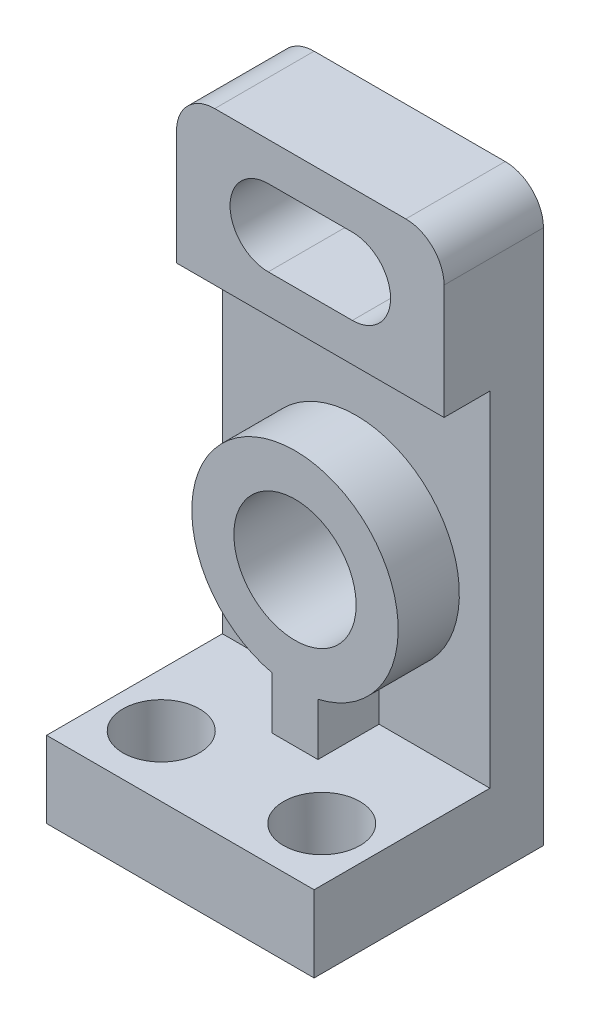
ISO-10303-21;
HEADER;
FILE_DESCRIPTION(('STEP AP214'),'2;1');
FILE_NAME('part.step','',(''),(''),'','','');
FILE_SCHEMA(('AUTOMOTIVE_DESIGN { 1 0 10303 214 1 1 1 1 }'));
ENDSEC;
DATA;
#1=APPLICATION_CONTEXT('core data for automotive mechanical design processes');
#2=APPLICATION_PROTOCOL_DEFINITION('international standard','automotive_design',2000,#1);
#3=PRODUCT_CONTEXT('',#1,'mechanical');
#4=PRODUCT('Part','Part','',(#3));
#5=PRODUCT_RELATED_PRODUCT_CATEGORY('part','',(#4));
#6=PRODUCT_DEFINITION_FORMATION('','',#4);
#7=PRODUCT_DEFINITION_CONTEXT('part definition',#1,'design');
#8=PRODUCT_DEFINITION('design','',#6,#7);
#9=PRODUCT_DEFINITION_SHAPE('','',#8);
#10=(LENGTH_UNIT() NAMED_UNIT(*) SI_UNIT(.MILLI.,.METRE.));
#11=(NAMED_UNIT(*) PLANE_ANGLE_UNIT() SI_UNIT($,.RADIAN.));
#12=(NAMED_UNIT(*) SI_UNIT($,.STERADIAN.) SOLID_ANGLE_UNIT());
#13=UNCERTAINTY_MEASURE_WITH_UNIT(LENGTH_MEASURE(1.E-05),#10,'distance_accuracy_value','');
#14=(GEOMETRIC_REPRESENTATION_CONTEXT(3) GLOBAL_UNCERTAINTY_ASSIGNED_CONTEXT((#13)) GLOBAL_UNIT_ASSIGNED_CONTEXT((#10,
#11,#12)) REPRESENTATION_CONTEXT('',''));
#15=CARTESIAN_POINT('',(0.,0.,0.));
#16=DIRECTION('',(0.,0.,1.));
#17=DIRECTION('',(1.,0.,0.));
#18=AXIS2_PLACEMENT_3D('',#15,#16,#17);
#19=CARTESIAN_POINT('',(17.5,10.,6.99999999999999));
#20=DIRECTION('',(0.,0.,-1.));
#21=DIRECTION('',(-1.,0.,0.));
#22=AXIS2_PLACEMENT_3D('',#19,#20,#21);
#23=PLANE('',#22);
#24=DIRECTION('',(0.,-1.,0.));
#25=VECTOR('',#24,1.);
#26=CARTESIAN_POINT('',(-3.,16.8375534189118,6.99999999999999));
#27=LINE('',#26,#25);
#28=CARTESIAN_POINT('',(-3.,16.8375534189118,6.99999999999999));
#29=VERTEX_POINT('',#28);
#30=CARTESIAN_POINT('',(-3.,10.,6.99999999999999));
#31=VERTEX_POINT('',#30);
#32=EDGE_CURVE('E211',#29,#31,#27,.T.);
#33=ORIENTED_EDGE('',*,*,#32,.F.);
#34=CARTESIAN_POINT('',(0.,30.,6.99999999999999));
#35=DIRECTION('',(0.,0.,1.));
#36=DIRECTION('',(1.,0.,0.));
#37=AXIS2_PLACEMENT_3D('',#34,#35,#36);
#38=CIRCLE('',#37,13.5);
#39=CARTESIAN_POINT('',(3.,16.8375534189118,6.99999999999999));
#40=VERTEX_POINT('',#39);
#41=EDGE_CURVE('E167',#40,#29,#38,.T.);
#42=ORIENTED_EDGE('',*,*,#41,.F.);
#43=DIRECTION('',(0.,1.,0.));
#44=VECTOR('',#43,1.);
#45=CARTESIAN_POINT('',(3.,16.8375534189118,6.99999999999999));
#46=LINE('',#45,#44);
#47=CARTESIAN_POINT('',(3.,10.,6.99999999999999));
#48=VERTEX_POINT('',#47);
#49=EDGE_CURVE('E203',#48,#40,#46,.T.);
#50=ORIENTED_EDGE('',*,*,#49,.F.);
#51=DIRECTION('',(-1.,0.,0.));
#52=VECTOR('',#51,1.);
#53=CARTESIAN_POINT('',(17.5,10.,6.99999999999999));
#54=LINE('',#53,#52);
#55=CARTESIAN_POINT('',(17.5,10.,6.99999999999999));
#56=VERTEX_POINT('',#55);
#57=EDGE_CURVE('E262',#56,#48,#54,.T.);
#58=ORIENTED_EDGE('',*,*,#57,.F.);
#59=DIRECTION('',(0.,-1.,0.));
#60=VECTOR('',#59,1.);
#61=CARTESIAN_POINT('',(17.5,10.,6.99999999999999));
#62=LINE('',#61,#60);
#63=CARTESIAN_POINT('',(17.5,55.,6.99999999999999));
#64=VERTEX_POINT('',#63);
#65=EDGE_CURVE('E235',#64,#56,#62,.T.);
#66=ORIENTED_EDGE('',*,*,#65,.F.);
#67=DIRECTION('',(-1.,0.,0.));
#68=VECTOR('',#67,1.);
#69=CARTESIAN_POINT('',(17.5,55.,6.99999999999999));
#70=LINE('',#69,#68);
#71=CARTESIAN_POINT('',(-17.5,55.,6.99999999999999));
#72=VERTEX_POINT('',#71);
#73=EDGE_CURVE('E270',#64,#72,#70,.T.);
#74=ORIENTED_EDGE('',*,*,#73,.T.);
#75=DIRECTION('',(0.,-1.,0.));
#76=VECTOR('',#75,1.);
#77=CARTESIAN_POINT('',(-17.5,10.,6.99999999999999));
#78=LINE('',#77,#76);
#79=CARTESIAN_POINT('',(-17.5,10.,6.99999999999999));
#80=VERTEX_POINT('',#79);
#81=EDGE_CURVE('E250',#72,#80,#78,.T.);
#82=ORIENTED_EDGE('',*,*,#81,.T.);
#83=EDGE_CURVE('E263',#31,#80,#54,.T.);
#84=ORIENTED_EDGE('',*,*,#83,.F.);
#85=EDGE_LOOP('',(#33,#42,#50,#58,#66,#74,#82,#84));
#86=FACE_BOUND('',#85,.T.);
#87=ADVANCED_FACE('F39',(#86),#23,.F.);
#88=CARTESIAN_POINT('',(17.5,10.,30.));
#89=DIRECTION('',(0.,-1.,0.));
#90=DIRECTION('',(0.,0.,-1.));
#91=AXIS2_PLACEMENT_3D('',#88,#89,#90);
#92=PLANE('',#91);
#93=CARTESIAN_POINT('',(-10.5,10.,22.));
#94=DIRECTION('',(0.,1.,0.));
#95=DIRECTION('',(0.,0.,1.));
#96=AXIS2_PLACEMENT_3D('',#93,#94,#95);
#97=CIRCLE('',#96,5.);
#98=CARTESIAN_POINT('',(-10.5,10.,27.));
#99=VERTEX_POINT('',#98);
#100=EDGE_CURVE('E314',#99,#99,#97,.T.);
#101=ORIENTED_EDGE('',*,*,#100,.F.);
#102=EDGE_LOOP('',(#101));
#103=FACE_BOUND('',#102,.T.);
#104=CARTESIAN_POINT('',(10.5,10.,22.));
#105=DIRECTION('',(0.,1.,0.));
#106=DIRECTION('',(0.,0.,-1.));
#107=AXIS2_PLACEMENT_3D('',#104,#105,#106);
#108=CIRCLE('',#107,5.);
#109=CARTESIAN_POINT('',(10.5,10.,17.));
#110=VERTEX_POINT('',#109);
#111=EDGE_CURVE('E312',#110,#110,#108,.T.);
#112=ORIENTED_EDGE('',*,*,#111,.F.);
#113=EDGE_LOOP('',(#112));
#114=FACE_BOUND('',#113,.T.);
#115=DIRECTION('',(0.,0.,-1.));
#116=VECTOR('',#115,1.);
#117=CARTESIAN_POINT('',(-3.,10.,15.));
#118=LINE('',#117,#116);
#119=CARTESIAN_POINT('',(-3.,10.,15.));
#120=VERTEX_POINT('',#119);
#121=EDGE_CURVE('E217',#120,#31,#118,.T.);
#122=ORIENTED_EDGE('',*,*,#121,.T.);
#123=ORIENTED_EDGE('',*,*,#83,.T.);
#124=DIRECTION('',(0.,0.,1.));
#125=VECTOR('',#124,1.);
#126=CARTESIAN_POINT('',(-17.5,10.,30.));
#127=LINE('',#126,#125);
#128=CARTESIAN_POINT('',(-17.5,10.,30.));
#129=VERTEX_POINT('',#128);
#130=EDGE_CURVE('E246',#80,#129,#127,.T.);
#131=ORIENTED_EDGE('',*,*,#130,.T.);
#132=DIRECTION('',(-1.,0.,0.));
#133=VECTOR('',#132,1.);
#134=CARTESIAN_POINT('',(17.5,10.,30.));
#135=LINE('',#134,#133);
#136=CARTESIAN_POINT('',(17.5,10.,30.));
#137=VERTEX_POINT('',#136);
#138=EDGE_CURVE('E257',#137,#129,#135,.T.);
#139=ORIENTED_EDGE('',*,*,#138,.F.);
#140=DIRECTION('',(0.,0.,1.));
#141=VECTOR('',#140,1.);
#142=CARTESIAN_POINT('',(17.5,10.,30.));
#143=LINE('',#142,#141);
#144=EDGE_CURVE('E234',#56,#137,#143,.T.);
#145=ORIENTED_EDGE('',*,*,#144,.F.);
#146=ORIENTED_EDGE('',*,*,#57,.T.);
#147=DIRECTION('',(0.,0.,-1.));
#148=VECTOR('',#147,1.);
#149=CARTESIAN_POINT('',(3.,10.,15.));
#150=LINE('',#149,#148);
#151=CARTESIAN_POINT('',(3.,10.,15.));
#152=VERTEX_POINT('',#151);
#153=EDGE_CURVE('E216',#152,#48,#150,.T.);
#154=ORIENTED_EDGE('',*,*,#153,.F.);
#155=DIRECTION('',(1.,0.,0.));
#156=VECTOR('',#155,1.);
#157=CARTESIAN_POINT('',(-3.,10.,15.));
#158=LINE('',#157,#156);
#159=EDGE_CURVE('E204',#120,#152,#158,.T.);
#160=ORIENTED_EDGE('',*,*,#159,.F.);
#161=EDGE_LOOP('',(#122,#123,#131,#139,#145,#146,#154,#160));
#162=FACE_BOUND('',#161,.T.);
#163=ADVANCED_FACE('F324',(#103,#114,#162),#92,.F.);
#164=CARTESIAN_POINT('',(17.5,75.,0.));
#165=DIRECTION('',(0.,0.,1.));
#166=DIRECTION('',(0.,-1.,0.));
#167=AXIS2_PLACEMENT_3D('',#164,#165,#166);
#168=PLANE('',#167);
#169=DIRECTION('',(1.,0.,0.));
#170=VECTOR('',#169,1.);
#171=CARTESIAN_POINT('',(-5.5,70.,0.));
#172=LINE('',#171,#170);
#173=CARTESIAN_POINT('',(-5.5,70.,0.));
#174=VERTEX_POINT('',#173);
#175=CARTESIAN_POINT('',(5.5,70.,0.));
#176=VERTEX_POINT('',#175);
#177=EDGE_CURVE('E179',#174,#176,#172,.T.);
#178=ORIENTED_EDGE('',*,*,#177,.F.);
#179=CARTESIAN_POINT('',(-5.5,65.,0.));
#180=DIRECTION('',(0.,0.,1.));
#181=DIRECTION('',(0.,-1.,0.));
#182=AXIS2_PLACEMENT_3D('',#179,#180,#181);
#183=CIRCLE('',#182,5.);
#184=CARTESIAN_POINT('',(-5.5,60.,0.));
#185=VERTEX_POINT('',#184);
#186=EDGE_CURVE('E170',#185,#174,#183,.F.);
#187=ORIENTED_EDGE('',*,*,#186,.F.);
#188=DIRECTION('',(-1.,0.,0.));
#189=VECTOR('',#188,1.);
#190=CARTESIAN_POINT('',(-5.5,60.,0.));
#191=LINE('',#190,#189);
#192=CARTESIAN_POINT('',(5.5,60.,0.));
#193=VERTEX_POINT('',#192);
#194=EDGE_CURVE('E161',#193,#185,#191,.T.);
#195=ORIENTED_EDGE('',*,*,#194,.F.);
#196=CARTESIAN_POINT('',(5.5,65.,0.));
#197=DIRECTION('',(0.,0.,1.));
#198=DIRECTION('',(0.,-1.,0.));
#199=AXIS2_PLACEMENT_3D('',#196,#197,#198);
#200=CIRCLE('',#199,5.);
#201=EDGE_CURVE('E182',#176,#193,#200,.F.);
#202=ORIENTED_EDGE('',*,*,#201,.F.);
#203=EDGE_LOOP('',(#178,#187,#195,#202));
#204=FACE_BOUND('',#203,.T.);
#205=CARTESIAN_POINT('',(0.,30.,0.));
#206=DIRECTION('',(0.,0.,1.));
#207=DIRECTION('',(0.,-1.,0.));
#208=AXIS2_PLACEMENT_3D('',#205,#206,#207);
#209=CIRCLE('',#208,8.);
#210=CARTESIAN_POINT('',(0.,22.,0.));
#211=VERTEX_POINT('',#210);
#212=EDGE_CURVE('E173',#211,#211,#209,.F.);
#213=ORIENTED_EDGE('',*,*,#212,.F.);
#214=EDGE_LOOP('',(#213));
#215=FACE_BOUND('',#214,.T.);
#216=DIRECTION('',(-1.,0.,0.));
#217=VECTOR('',#216,1.);
#218=CARTESIAN_POINT('',(17.5,75.,0.));
#219=LINE('',#218,#217);
#220=CARTESIAN_POINT('',(12.5,75.,0.));
#221=VERTEX_POINT('',#220);
#222=CARTESIAN_POINT('',(-12.5,75.,0.));
#223=VERTEX_POINT('',#222);
#224=EDGE_CURVE('E277',#221,#223,#219,.T.);
#225=ORIENTED_EDGE('',*,*,#224,.F.);
#226=CARTESIAN_POINT('',(12.5,70.,0.));
#227=DIRECTION('',(0.,0.,1.));
#228=DIRECTION('',(0.,-1.,0.));
#229=AXIS2_PLACEMENT_3D('',#226,#227,#228);
#230=CIRCLE('',#229,5.);
#231=CARTESIAN_POINT('',(17.5,70.,0.));
#232=VERTEX_POINT('',#231);
#233=EDGE_CURVE('E291',#221,#232,#230,.F.);
#234=ORIENTED_EDGE('',*,*,#233,.T.);
#235=DIRECTION('',(0.,1.,0.));
#236=VECTOR('',#235,1.);
#237=CARTESIAN_POINT('',(17.5,75.,0.));
#238=LINE('',#237,#236);
#239=CARTESIAN_POINT('',(17.5,0.,0.));
#240=VERTEX_POINT('',#239);
#241=EDGE_CURVE('E221',#240,#232,#238,.T.);
#242=ORIENTED_EDGE('',*,*,#241,.F.);
#243=DIRECTION('',(-1.,0.,0.));
#244=VECTOR('',#243,1.);
#245=CARTESIAN_POINT('',(17.5,0.,0.));
#246=LINE('',#245,#244);
#247=CARTESIAN_POINT('',(-17.5,0.,0.));
#248=VERTEX_POINT('',#247);
#249=EDGE_CURVE('E238',#240,#248,#246,.T.);
#250=ORIENTED_EDGE('',*,*,#249,.T.);
#251=DIRECTION('',(0.,1.,0.));
#252=VECTOR('',#251,1.);
#253=CARTESIAN_POINT('',(-17.5,75.,0.));
#254=LINE('',#253,#252);
#255=CARTESIAN_POINT('',(-17.5,70.,0.));
#256=VERTEX_POINT('',#255);
#257=EDGE_CURVE('E224',#248,#256,#254,.T.);
#258=ORIENTED_EDGE('',*,*,#257,.T.);
#259=CARTESIAN_POINT('',(-12.5,70.,0.));
#260=DIRECTION('',(0.,0.,1.));
#261=DIRECTION('',(0.,-1.,0.));
#262=AXIS2_PLACEMENT_3D('',#259,#260,#261);
#263=CIRCLE('',#262,5.);
#264=EDGE_CURVE('E292',#256,#223,#263,.F.);
#265=ORIENTED_EDGE('',*,*,#264,.T.);
#266=EDGE_LOOP('',(#225,#234,#242,#250,#258,#265));
#267=FACE_BOUND('',#266,.T.);
#268=ADVANCED_FACE('F180',(#204,#215,#267),#168,.F.);
#269=CARTESIAN_POINT('',(17.5,75.,13.));
#270=DIRECTION('',(0.,-1.,0.));
#271=DIRECTION('',(0.,0.,-1.));
#272=AXIS2_PLACEMENT_3D('',#269,#270,#271);
#273=PLANE('',#272);
#274=DIRECTION('',(-1.,0.,0.));
#275=VECTOR('',#274,1.);
#276=CARTESIAN_POINT('',(17.5,75.,13.));
#277=LINE('',#276,#275);
#278=CARTESIAN_POINT('',(12.5,75.,13.));
#279=VERTEX_POINT('',#278);
#280=CARTESIAN_POINT('',(-12.5,75.,13.));
#281=VERTEX_POINT('',#280);
#282=EDGE_CURVE('E272',#279,#281,#277,.T.);
#283=ORIENTED_EDGE('',*,*,#282,.F.);
#284=DIRECTION('',(0.,0.,1.));
#285=VECTOR('',#284,1.);
#286=CARTESIAN_POINT('',(12.5,75.,13.));
#287=LINE('',#286,#285);
#288=EDGE_CURVE('E289',#279,#221,#287,.F.);
#289=ORIENTED_EDGE('',*,*,#288,.T.);
#290=ORIENTED_EDGE('',*,*,#224,.T.);
#291=DIRECTION('',(0.,0.,1.));
#292=VECTOR('',#291,1.);
#293=CARTESIAN_POINT('',(-12.5,75.,13.));
#294=LINE('',#293,#292);
#295=EDGE_CURVE('E287',#223,#281,#294,.T.);
#296=ORIENTED_EDGE('',*,*,#295,.T.);
#297=EDGE_LOOP('',(#283,#289,#290,#296));
#298=FACE_BOUND('',#297,.T.);
#299=ADVANCED_FACE('F392',(#298),#273,.F.);
#300=CARTESIAN_POINT('',(17.5,55.,13.));
#301=DIRECTION('',(0.,0.,-1.));
#302=DIRECTION('',(-1.,0.,0.));
#303=AXIS2_PLACEMENT_3D('',#300,#301,#302);
#304=PLANE('',#303);
#305=DIRECTION('',(-1.,0.,0.));
#306=VECTOR('',#305,1.);
#307=CARTESIAN_POINT('',(17.5,60.,13.));
#308=LINE('',#307,#306);
#309=CARTESIAN_POINT('',(5.5,60.,13.));
#310=VERTEX_POINT('',#309);
#311=CARTESIAN_POINT('',(-5.5,60.,13.));
#312=VERTEX_POINT('',#311);
#313=EDGE_CURVE('E297',#310,#312,#308,.T.);
#314=ORIENTED_EDGE('',*,*,#313,.T.);
#315=CARTESIAN_POINT('',(-5.5,65.,13.));
#316=DIRECTION('',(0.,0.,-1.));
#317=DIRECTION('',(-1.,0.,0.));
#318=AXIS2_PLACEMENT_3D('',#315,#316,#317);
#319=CIRCLE('',#318,5.);
#320=CARTESIAN_POINT('',(-5.5,70.,13.));
#321=VERTEX_POINT('',#320);
#322=EDGE_CURVE('E11',#312,#321,#319,.T.);
#323=ORIENTED_EDGE('',*,*,#322,.T.);
#324=DIRECTION('',(1.,0.,0.));
#325=VECTOR('',#324,1.);
#326=CARTESIAN_POINT('',(17.5,70.,13.));
#327=LINE('',#326,#325);
#328=CARTESIAN_POINT('',(5.5,70.,13.));
#329=VERTEX_POINT('',#328);
#330=EDGE_CURVE('E50',#321,#329,#327,.T.);
#331=ORIENTED_EDGE('',*,*,#330,.T.);
#332=CARTESIAN_POINT('',(5.5,65.,13.));
#333=DIRECTION('',(0.,0.,-1.));
#334=DIRECTION('',(-1.,0.,0.));
#335=AXIS2_PLACEMENT_3D('',#332,#333,#334);
#336=CIRCLE('',#335,5.);
#337=EDGE_CURVE('E298',#329,#310,#336,.T.);
#338=ORIENTED_EDGE('',*,*,#337,.T.);
#339=EDGE_LOOP('',(#314,#323,#331,#338));
#340=FACE_BOUND('',#339,.T.);
#341=DIRECTION('',(0.,-1.,0.));
#342=VECTOR('',#341,1.);
#343=CARTESIAN_POINT('',(17.5,55.,13.));
#344=LINE('',#343,#342);
#345=CARTESIAN_POINT('',(17.5,70.,13.));
#346=VERTEX_POINT('',#345);
#347=CARTESIAN_POINT('',(17.5,55.,13.));
#348=VERTEX_POINT('',#347);
#349=EDGE_CURVE('E227',#346,#348,#344,.T.);
#350=ORIENTED_EDGE('',*,*,#349,.F.);
#351=CARTESIAN_POINT('',(12.5,70.,13.));
#352=DIRECTION('',(0.,0.,-1.));
#353=DIRECTION('',(-1.,0.,0.));
#354=AXIS2_PLACEMENT_3D('',#351,#352,#353);
#355=CIRCLE('',#354,5.);
#356=EDGE_CURVE('E283',#346,#279,#355,.F.);
#357=ORIENTED_EDGE('',*,*,#356,.T.);
#358=ORIENTED_EDGE('',*,*,#282,.T.);
#359=CARTESIAN_POINT('',(-12.5,70.,13.));
#360=DIRECTION('',(0.,0.,-1.));
#361=DIRECTION('',(-1.,0.,0.));
#362=AXIS2_PLACEMENT_3D('',#359,#360,#361);
#363=CIRCLE('',#362,5.);
#364=CARTESIAN_POINT('',(-17.5,70.,13.));
#365=VERTEX_POINT('',#364);
#366=EDGE_CURVE('E282',#281,#365,#363,.F.);
#367=ORIENTED_EDGE('',*,*,#366,.T.);
#368=DIRECTION('',(0.,-1.,0.));
#369=VECTOR('',#368,1.);
#370=CARTESIAN_POINT('',(-17.5,55.,13.));
#371=LINE('',#370,#369);
#372=CARTESIAN_POINT('',(-17.5,55.,13.));
#373=VERTEX_POINT('',#372);
#374=EDGE_CURVE('E244',#365,#373,#371,.T.);
#375=ORIENTED_EDGE('',*,*,#374,.T.);
#376=DIRECTION('',(-1.,0.,0.));
#377=VECTOR('',#376,1.);
#378=CARTESIAN_POINT('',(17.5,55.,13.));
#379=LINE('',#378,#377);
#380=EDGE_CURVE('E269',#348,#373,#379,.T.);
#381=ORIENTED_EDGE('',*,*,#380,.F.);
#382=EDGE_LOOP('',(#350,#357,#358,#367,#375,#381));
#383=FACE_BOUND('',#382,.T.);
#384=ADVANCED_FACE('F303',(#340,#383),#304,.F.);
#385=CARTESIAN_POINT('',(17.5,55.,6.99999999999999));
#386=DIRECTION('',(0.,1.,0.));
#387=DIRECTION('',(0.,0.,1.));
#388=AXIS2_PLACEMENT_3D('',#385,#386,#387);
#389=PLANE('',#388);
#390=DIRECTION('',(0.,0.,-1.));
#391=VECTOR('',#390,1.);
#392=CARTESIAN_POINT('',(-17.5,55.,6.99999999999999));
#393=LINE('',#392,#391);
#394=EDGE_CURVE('E245',#373,#72,#393,.T.);
#395=ORIENTED_EDGE('',*,*,#394,.T.);
#396=ORIENTED_EDGE('',*,*,#73,.F.);
#397=DIRECTION('',(0.,0.,-1.));
#398=VECTOR('',#397,1.);
#399=CARTESIAN_POINT('',(17.5,55.,6.99999999999999));
#400=LINE('',#399,#398);
#401=EDGE_CURVE('E230',#348,#64,#400,.T.);
#402=ORIENTED_EDGE('',*,*,#401,.F.);
#403=ORIENTED_EDGE('',*,*,#380,.T.);
#404=EDGE_LOOP('',(#395,#396,#402,#403));
#405=FACE_BOUND('',#404,.T.);
#406=ADVANCED_FACE('F387',(#405),#389,.F.);
#407=CARTESIAN_POINT('',(17.5,0.,30.));
#408=DIRECTION('',(0.,0.,-1.));
#409=DIRECTION('',(-1.,0.,0.));
#410=AXIS2_PLACEMENT_3D('',#407,#408,#409);
#411=PLANE('',#410);
#412=DIRECTION('',(0.,-1.,0.));
#413=VECTOR('',#412,1.);
#414=CARTESIAN_POINT('',(-17.5,0.,30.));
#415=LINE('',#414,#413);
#416=CARTESIAN_POINT('',(-17.5,0.,30.));
#417=VERTEX_POINT('',#416);
#418=EDGE_CURVE('E252',#129,#417,#415,.T.);
#419=ORIENTED_EDGE('',*,*,#418,.T.);
#420=DIRECTION('',(-1.,0.,0.));
#421=VECTOR('',#420,1.);
#422=CARTESIAN_POINT('',(17.5,0.,30.));
#423=LINE('',#422,#421);
#424=CARTESIAN_POINT('',(17.5,0.,30.));
#425=VERTEX_POINT('',#424);
#426=EDGE_CURVE('E260',#425,#417,#423,.T.);
#427=ORIENTED_EDGE('',*,*,#426,.F.);
#428=DIRECTION('',(0.,-1.,0.));
#429=VECTOR('',#428,1.);
#430=CARTESIAN_POINT('',(17.5,0.,30.));
#431=LINE('',#430,#429);
#432=EDGE_CURVE('E237',#137,#425,#431,.T.);
#433=ORIENTED_EDGE('',*,*,#432,.F.);
#434=ORIENTED_EDGE('',*,*,#138,.T.);
#435=EDGE_LOOP('',(#419,#427,#433,#434));
#436=FACE_BOUND('',#435,.T.);
#437=ADVANCED_FACE('F352',(#436),#411,.F.);
#438=CARTESIAN_POINT('',(17.5,0.,0.));
#439=DIRECTION('',(0.,1.,0.));
#440=DIRECTION('',(0.,0.,1.));
#441=AXIS2_PLACEMENT_3D('',#438,#439,#440);
#442=PLANE('',#441);
#443=CARTESIAN_POINT('',(-10.5,0.,22.));
#444=DIRECTION('',(0.,1.,0.));
#445=DIRECTION('',(0.,0.,1.));
#446=AXIS2_PLACEMENT_3D('',#443,#444,#445);
#447=CIRCLE('',#446,5.);
#448=CARTESIAN_POINT('',(-10.5,0.,27.));
#449=VERTEX_POINT('',#448);
#450=EDGE_CURVE('E194',#449,#449,#447,.F.);
#451=ORIENTED_EDGE('',*,*,#450,.F.);
#452=EDGE_LOOP('',(#451));
#453=FACE_BOUND('',#452,.T.);
#454=CARTESIAN_POINT('',(10.5,0.,22.));
#455=DIRECTION('',(0.,1.,0.));
#456=DIRECTION('',(0.,0.,1.));
#457=AXIS2_PLACEMENT_3D('',#454,#455,#456);
#458=CIRCLE('',#457,5.);
#459=CARTESIAN_POINT('',(10.5,0.,27.));
#460=VERTEX_POINT('',#459);
#461=EDGE_CURVE('E313',#460,#460,#458,.F.);
#462=ORIENTED_EDGE('',*,*,#461,.F.);
#463=EDGE_LOOP('',(#462));
#464=FACE_BOUND('',#463,.T.);
#465=DIRECTION('',(0.,0.,-1.));
#466=VECTOR('',#465,1.);
#467=CARTESIAN_POINT('',(-17.5,0.,0.));
#468=LINE('',#467,#466);
#469=EDGE_CURVE('E229',#417,#248,#468,.T.);
#470=ORIENTED_EDGE('',*,*,#469,.T.);
#471=ORIENTED_EDGE('',*,*,#249,.F.);
#472=DIRECTION('',(0.,0.,-1.));
#473=VECTOR('',#472,1.);
#474=CARTESIAN_POINT('',(17.5,0.,0.));
#475=LINE('',#474,#473);
#476=EDGE_CURVE('E236',#425,#240,#475,.T.);
#477=ORIENTED_EDGE('',*,*,#476,.F.);
#478=ORIENTED_EDGE('',*,*,#426,.T.);
#479=EDGE_LOOP('',(#470,#471,#477,#478));
#480=FACE_BOUND('',#479,.T.);
#481=ADVANCED_FACE('F419',(#453,#464,#480),#442,.F.);
#482=CARTESIAN_POINT('',(17.5,0.,0.));
#483=DIRECTION('',(-1.,0.,0.));
#484=DIRECTION('',(0.,0.,1.));
#485=AXIS2_PLACEMENT_3D('',#482,#483,#484);
#486=PLANE('',#485);
#487=ORIENTED_EDGE('',*,*,#241,.T.);
#488=DIRECTION('',(0.,0.,1.));
#489=VECTOR('',#488,1.);
#490=CARTESIAN_POINT('',(17.5,70.,0.));
#491=LINE('',#490,#489);
#492=EDGE_CURVE('E276',#232,#346,#491,.T.);
#493=ORIENTED_EDGE('',*,*,#492,.T.);
#494=ORIENTED_EDGE('',*,*,#349,.T.);
#495=ORIENTED_EDGE('',*,*,#401,.T.);
#496=ORIENTED_EDGE('',*,*,#65,.T.);
#497=ORIENTED_EDGE('',*,*,#144,.T.);
#498=ORIENTED_EDGE('',*,*,#432,.T.);
#499=ORIENTED_EDGE('',*,*,#476,.T.);
#500=EDGE_LOOP('',(#487,#493,#494,#495,#496,#497,#498,#499));
#501=FACE_BOUND('',#500,.T.);
#502=ADVANCED_FACE('F357',(#501),#486,.F.);
#503=CARTESIAN_POINT('',(-17.5,0.,0.));
#504=DIRECTION('',(-1.,0.,0.));
#505=DIRECTION('',(0.,0.,1.));
#506=AXIS2_PLACEMENT_3D('',#503,#504,#505);
#507=PLANE('',#506);
#508=ORIENTED_EDGE('',*,*,#374,.F.);
#509=DIRECTION('',(0.,0.,1.));
#510=VECTOR('',#509,1.);
#511=CARTESIAN_POINT('',(-17.5,70.,0.));
#512=LINE('',#511,#510);
#513=EDGE_CURVE('E293',#365,#256,#512,.F.);
#514=ORIENTED_EDGE('',*,*,#513,.T.);
#515=ORIENTED_EDGE('',*,*,#257,.F.);
#516=ORIENTED_EDGE('',*,*,#469,.F.);
#517=ORIENTED_EDGE('',*,*,#418,.F.);
#518=ORIENTED_EDGE('',*,*,#130,.F.);
#519=ORIENTED_EDGE('',*,*,#81,.F.);
#520=ORIENTED_EDGE('',*,*,#394,.F.);
#521=EDGE_LOOP('',(#508,#514,#515,#516,#517,#518,#519,#520));
#522=FACE_BOUND('',#521,.T.);
#523=ADVANCED_FACE('F347',(#522),#507,.T.);
#524=CARTESIAN_POINT('',(12.5,70.,0.));
#525=DIRECTION('',(0.,0.,1.));
#526=DIRECTION('',(1.,0.,0.));
#527=AXIS2_PLACEMENT_3D('',#524,#525,#526);
#528=CYLINDRICAL_SURFACE('',#527,5.);
#529=ORIENTED_EDGE('',*,*,#233,.F.);
#530=ORIENTED_EDGE('',*,*,#288,.F.);
#531=ORIENTED_EDGE('',*,*,#356,.F.);
#532=ORIENTED_EDGE('',*,*,#492,.F.);
#533=EDGE_LOOP('',(#529,#530,#531,#532));
#534=FACE_BOUND('',#533,.T.);
#535=ADVANCED_FACE('F400',(#534),#528,.T.);
#536=CARTESIAN_POINT('',(-12.5,70.,13.));
#537=DIRECTION('',(0.,0.,-1.));
#538=DIRECTION('',(-1.,0.,0.));
#539=AXIS2_PLACEMENT_3D('',#536,#537,#538);
#540=CYLINDRICAL_SURFACE('',#539,5.);
#541=ORIENTED_EDGE('',*,*,#264,.F.);
#542=ORIENTED_EDGE('',*,*,#513,.F.);
#543=ORIENTED_EDGE('',*,*,#366,.F.);
#544=ORIENTED_EDGE('',*,*,#295,.F.);
#545=EDGE_LOOP('',(#541,#542,#543,#544));
#546=FACE_BOUND('',#545,.T.);
#547=ADVANCED_FACE('F41',(#546),#540,.T.);
#548=CARTESIAN_POINT('',(0.,30.,15.));
#549=DIRECTION('',(0.,0.,-1.));
#550=DIRECTION('',(-1.,0.,0.));
#551=AXIS2_PLACEMENT_3D('',#548,#549,#550);
#552=CYLINDRICAL_SURFACE('',#551,13.5);
#553=ORIENTED_EDGE('',*,*,#41,.T.);
#554=DIRECTION('',(0.,0.,-1.));
#555=VECTOR('',#554,1.);
#556=CARTESIAN_POINT('',(-3.,16.8375534189118,15.));
#557=LINE('',#556,#555);
#558=CARTESIAN_POINT('',(-3.,16.8375534189118,15.));
#559=VERTEX_POINT('',#558);
#560=EDGE_CURVE('E222',#559,#29,#557,.T.);
#561=ORIENTED_EDGE('',*,*,#560,.F.);
#562=CARTESIAN_POINT('',(0.,30.,15.));
#563=DIRECTION('',(0.,0.,1.));
#564=DIRECTION('',(1.,0.,0.));
#565=AXIS2_PLACEMENT_3D('',#562,#563,#564);
#566=CIRCLE('',#565,13.5);
#567=CARTESIAN_POINT('',(3.,16.8375534189118,15.));
#568=VERTEX_POINT('',#567);
#569=EDGE_CURVE('E197',#568,#559,#566,.T.);
#570=ORIENTED_EDGE('',*,*,#569,.F.);
#571=DIRECTION('',(0.,0.,-1.));
#572=VECTOR('',#571,1.);
#573=CARTESIAN_POINT('',(3.,16.8375534189118,15.));
#574=LINE('',#573,#572);
#575=EDGE_CURVE('E208',#568,#40,#574,.T.);
#576=ORIENTED_EDGE('',*,*,#575,.T.);
#577=EDGE_LOOP('',(#553,#561,#570,#576));
#578=FACE_BOUND('',#577,.T.);
#579=ADVANCED_FACE('F368',(#578),#552,.T.);
#580=CARTESIAN_POINT('',(-3.,16.8375534189118,15.));
#581=DIRECTION('',(1.,0.,0.));
#582=DIRECTION('',(0.,1.,0.));
#583=AXIS2_PLACEMENT_3D('',#580,#581,#582);
#584=PLANE('',#583);
#585=ORIENTED_EDGE('',*,*,#32,.T.);
#586=ORIENTED_EDGE('',*,*,#121,.F.);
#587=DIRECTION('',(0.,-1.,0.));
#588=VECTOR('',#587,1.);
#589=CARTESIAN_POINT('',(-3.,16.8375534189118,15.));
#590=LINE('',#589,#588);
#591=EDGE_CURVE('E199',#559,#120,#590,.T.);
#592=ORIENTED_EDGE('',*,*,#591,.F.);
#593=ORIENTED_EDGE('',*,*,#560,.T.);
#594=EDGE_LOOP('',(#585,#586,#592,#593));
#595=FACE_BOUND('',#594,.T.);
#596=ADVANCED_FACE('F367',(#595),#584,.F.);
#597=CARTESIAN_POINT('',(3.,16.8375534189118,15.));
#598=DIRECTION('',(-1.,0.,0.));
#599=DIRECTION('',(0.,-1.,0.));
#600=AXIS2_PLACEMENT_3D('',#597,#598,#599);
#601=PLANE('',#600);
#602=ORIENTED_EDGE('',*,*,#49,.T.);
#603=ORIENTED_EDGE('',*,*,#575,.F.);
#604=DIRECTION('',(0.,1.,0.));
#605=VECTOR('',#604,1.);
#606=CARTESIAN_POINT('',(3.,16.8375534189118,15.));
#607=LINE('',#606,#605);
#608=EDGE_CURVE('E206',#152,#568,#607,.T.);
#609=ORIENTED_EDGE('',*,*,#608,.F.);
#610=ORIENTED_EDGE('',*,*,#153,.T.);
#611=EDGE_LOOP('',(#602,#603,#609,#610));
#612=FACE_BOUND('',#611,.T.);
#613=ADVANCED_FACE('F362',(#612),#601,.F.);
#614=CARTESIAN_POINT('',(0.,30.,15.));
#615=DIRECTION('',(0.,0.,1.));
#616=DIRECTION('',(1.,0.,0.));
#617=AXIS2_PLACEMENT_3D('',#614,#615,#616);
#618=PLANE('',#617);
#619=CARTESIAN_POINT('',(0.,30.,15.));
#620=DIRECTION('',(0.,0.,1.));
#621=DIRECTION('',(1.,0.,0.));
#622=AXIS2_PLACEMENT_3D('',#619,#620,#621);
#623=CIRCLE('',#622,8.);
#624=CARTESIAN_POINT('',(8.,30.,15.));
#625=VERTEX_POINT('',#624);
#626=EDGE_CURVE('E192',#625,#625,#623,.T.);
#627=ORIENTED_EDGE('',*,*,#626,.F.);
#628=EDGE_LOOP('',(#627));
#629=FACE_BOUND('',#628,.T.);
#630=ORIENTED_EDGE('',*,*,#569,.T.);
#631=ORIENTED_EDGE('',*,*,#591,.T.);
#632=ORIENTED_EDGE('',*,*,#159,.T.);
#633=ORIENTED_EDGE('',*,*,#608,.T.);
#634=EDGE_LOOP('',(#630,#631,#632,#633));
#635=FACE_BOUND('',#634,.T.);
#636=ADVANCED_FACE('F369',(#629,#635),#618,.T.);
#637=CARTESIAN_POINT('',(0.,30.,-23.259406699226));
#638=DIRECTION('',(0.,0.,1.));
#639=DIRECTION('',(1.,0.,0.));
#640=AXIS2_PLACEMENT_3D('',#637,#638,#639);
#641=CYLINDRICAL_SURFACE('',#640,8.);
#642=ORIENTED_EDGE('',*,*,#212,.T.);
#643=EDGE_LOOP('',(#642));
#644=FACE_BOUND('',#643,.T.);
#645=ORIENTED_EDGE('',*,*,#626,.T.);
#646=EDGE_LOOP('',(#645));
#647=FACE_BOUND('',#646,.T.);
#648=ADVANCED_FACE('F452',(#644,#647),#641,.F.);
#649=CARTESIAN_POINT('',(-5.5,65.,-23.259406699226));
#650=DIRECTION('',(0.,0.,1.));
#651=DIRECTION('',(1.,0.,0.));
#652=AXIS2_PLACEMENT_3D('',#649,#650,#651);
#653=CYLINDRICAL_SURFACE('',#652,5.);
#654=DIRECTION('',(0.,0.,1.));
#655=VECTOR('',#654,1.);
#656=CARTESIAN_POINT('',(-5.5,60.,-23.259406699226));
#657=LINE('',#656,#655);
#658=EDGE_CURVE('E56',#185,#312,#657,.T.);
#659=ORIENTED_EDGE('',*,*,#658,.F.);
#660=ORIENTED_EDGE('',*,*,#186,.T.);
#661=DIRECTION('',(0.,0.,1.));
#662=VECTOR('',#661,1.);
#663=CARTESIAN_POINT('',(-5.5,70.,-23.259406699226));
#664=LINE('',#663,#662);
#665=EDGE_CURVE('E183',#174,#321,#664,.T.);
#666=ORIENTED_EDGE('',*,*,#665,.T.);
#667=ORIENTED_EDGE('',*,*,#322,.F.);
#668=EDGE_LOOP('',(#659,#660,#666,#667));
#669=FACE_BOUND('',#668,.T.);
#670=ADVANCED_FACE('F168',(#669),#653,.F.);
#671=CARTESIAN_POINT('',(-5.5,70.,-23.259406699226));
#672=DIRECTION('',(0.,1.,0.));
#673=DIRECTION('',(0.,0.,1.));
#674=AXIS2_PLACEMENT_3D('',#671,#672,#673);
#675=PLANE('',#674);
#676=ORIENTED_EDGE('',*,*,#665,.F.);
#677=ORIENTED_EDGE('',*,*,#177,.T.);
#678=DIRECTION('',(0.,0.,1.));
#679=VECTOR('',#678,1.);
#680=CARTESIAN_POINT('',(5.5,70.,-23.259406699226));
#681=LINE('',#680,#679);
#682=EDGE_CURVE('E187',#176,#329,#681,.T.);
#683=ORIENTED_EDGE('',*,*,#682,.T.);
#684=ORIENTED_EDGE('',*,*,#330,.F.);
#685=EDGE_LOOP('',(#676,#677,#683,#684));
#686=FACE_BOUND('',#685,.T.);
#687=ADVANCED_FACE('F308',(#686),#675,.F.);
#688=CARTESIAN_POINT('',(5.5,65.,-23.259406699226));
#689=DIRECTION('',(0.,0.,1.));
#690=DIRECTION('',(1.,0.,0.));
#691=AXIS2_PLACEMENT_3D('',#688,#689,#690);
#692=CYLINDRICAL_SURFACE('',#691,5.);
#693=ORIENTED_EDGE('',*,*,#682,.F.);
#694=ORIENTED_EDGE('',*,*,#201,.T.);
#695=DIRECTION('',(0.,0.,1.));
#696=VECTOR('',#695,1.);
#697=CARTESIAN_POINT('',(5.5,60.,-23.259406699226));
#698=LINE('',#697,#696);
#699=EDGE_CURVE('E53',#193,#310,#698,.T.);
#700=ORIENTED_EDGE('',*,*,#699,.T.);
#701=ORIENTED_EDGE('',*,*,#337,.F.);
#702=EDGE_LOOP('',(#693,#694,#700,#701));
#703=FACE_BOUND('',#702,.T.);
#704=ADVANCED_FACE('F310',(#703),#692,.F.);
#705=CARTESIAN_POINT('',(-5.5,60.,-23.259406699226));
#706=DIRECTION('',(0.,-1.,0.));
#707=DIRECTION('',(0.,0.,-1.));
#708=AXIS2_PLACEMENT_3D('',#705,#706,#707);
#709=PLANE('',#708);
#710=ORIENTED_EDGE('',*,*,#699,.F.);
#711=ORIENTED_EDGE('',*,*,#194,.T.);
#712=ORIENTED_EDGE('',*,*,#658,.T.);
#713=ORIENTED_EDGE('',*,*,#313,.F.);
#714=EDGE_LOOP('',(#710,#711,#712,#713));
#715=FACE_BOUND('',#714,.T.);
#716=ADVANCED_FACE('F165',(#715),#709,.F.);
#717=CARTESIAN_POINT('',(10.5,-14.142135623731,22.));
#718=DIRECTION('',(0.,1.,0.));
#719=DIRECTION('',(0.,0.,1.));
#720=AXIS2_PLACEMENT_3D('',#717,#718,#719);
#721=CYLINDRICAL_SURFACE('',#720,5.);
#722=ORIENTED_EDGE('',*,*,#461,.T.);
#723=EDGE_LOOP('',(#722));
#724=FACE_BOUND('',#723,.T.);
#725=ORIENTED_EDGE('',*,*,#111,.T.);
#726=EDGE_LOOP('',(#725));
#727=FACE_BOUND('',#726,.T.);
#728=ADVANCED_FACE('F432',(#724,#727),#721,.F.);
#729=CARTESIAN_POINT('',(-10.5,-14.142135623731,22.));
#730=DIRECTION('',(0.,1.,0.));
#731=DIRECTION('',(0.,0.,1.));
#732=AXIS2_PLACEMENT_3D('',#729,#730,#731);
#733=CYLINDRICAL_SURFACE('',#732,5.);
#734=ORIENTED_EDGE('',*,*,#450,.T.);
#735=EDGE_LOOP('',(#734));
#736=FACE_BOUND('',#735,.T.);
#737=ORIENTED_EDGE('',*,*,#100,.T.);
#738=EDGE_LOOP('',(#737));
#739=FACE_BOUND('',#738,.T.);
#740=ADVANCED_FACE('F323',(#736,#739),#733,.F.);
#741=CLOSED_SHELL('',(#87,#163,#268,#299,#384,#406,#437,#481,#502,#523,#535,#547,#579,#596,#613,
#636,#648,#670,#687,#704,#716,#728,#740));
#742=MANIFOLD_SOLID_BREP('B2',#741);
#743=ADVANCED_BREP_SHAPE_REPRESENTATION('',(#18,#742),#14);
#744=SHAPE_DEFINITION_REPRESENTATION(#9,#743);
ENDSEC;
END-ISO-10303-21;
